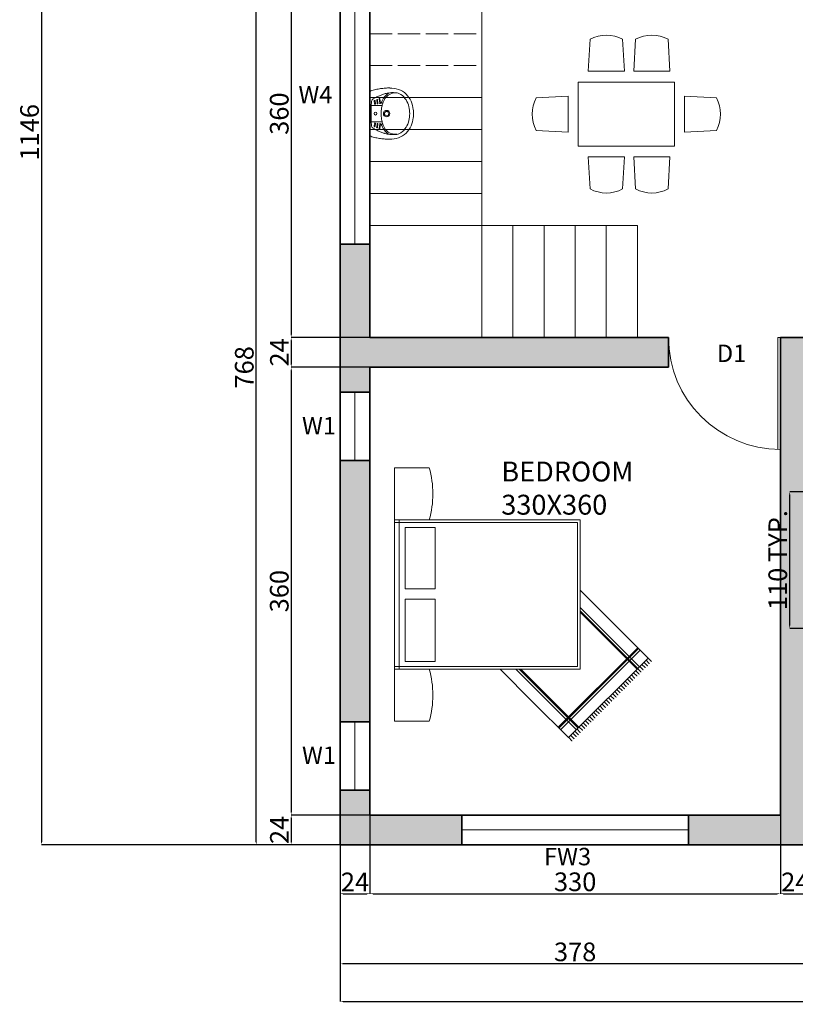
# Model space of a CAD drawing. Units: centimetres. Extents: x 2449 to 7478, y 778 to 2486.
# Tile 1 of 9: x 2449 to 3072, y 940 to 1732. Entities that reach past the tile are written whole.
import ezdxf

# ---------------------------------------------------------------- set-up
doc = ezdxf.new("R2010")
doc.units = ezdxf.units.CM
doc.linetypes.add('ACAD_ISO02W100', pattern=[15, 12, -3])
for name, color, linetype, lineweight in [('0.15', 34, 'Continuous', 15), ('A-ANNO-DIMS', 2, 'Continuous', 18), ('A-ANNO-TEXT', 7, 'Continuous', 18), ('A-AREA-IDEN', 7, 'Continuous', 18), ('A-DOOR', 4, 'Continuous', 18), ('A-FLOR-FIXT', 8, 'Continuous', 18), ('A-FLOR-STRS', 7, 'Continuous', 18), ('A-FLOR-STRS-OVHD', 7, 'ACAD_ISO02W100', 13), ('A-WALL', 7, 'Continuous', 35), ('A-WALL-PATT', 7, 'Continuous', 13), ('B-FURNITURE', 22, 'Continuous', 18), ('Win', 1, 'Continuous', 18)]:
    doc.layers.add(name, color=color, linetype=linetype, lineweight=lineweight)
doc.styles.get("Standard").update_dxf_attribs({"font": 'arial.ttf'})
doc.dimstyles.new('ISO-25', dxfattribs={"dimtxt": 15, "dimasz": 2.5, "dimexe": 0, "dimexo": 0, "dimgap": 0, "dimtad": 1, "dimtxsty": 'Standard', "dimcen": 2.5, "dimadec": 0, "dimazin": 0, "dimtfac": 1, "dimtmove": 0, "dimatfit": 3, "dimfxl": 1, "dimarcsym": 0})

# ---------------------------------------------------------------- blocks, each defined once
blk = doc.blocks.new('table-11')
at = {"color": 0, "linetype": 'ByBlock'}
for p, q in [((-1.122, 0.533), (-1.144, 0.134)), ((-0.716, 0.533), (-0.694, 0.134)), ((-0.554, 0.533), (-0.576, 0.134)), ((-0.148, 0.533), (-0.126, 0.134)), ((-1.144, 0.134), (-0.694, 0.134)), ((-0.576, 0.134), (-0.126, 0.134)), ((0, 0), (-1.2, 0)), ((-1.2, -0.8), (-1.2, 0)), ((0, -0.8), (0, 0)), ((-1.723, -0.197), (-1.324, -0.175)), ((-1.324, -0.625), (-1.324, -0.175)), ((0.523, -0.197), (0.124, -0.175)), ((0.124, -0.625), (0.124, -0.175)), ((-1.723, -0.603), (-1.324, -0.625)), ((0.523, -0.603), (0.124, -0.625)), ((0, -0.8), (-1.2, -0.8)), ((-1.144, -0.934), (-0.694, -0.934)), ((-1.122, -1.333), (-1.144, -0.934)), ((-0.716, -1.333), (-0.694, -0.934)), ((-0.576, -0.934), (-0.126, -0.934)), ((-0.554, -1.333), (-0.576, -0.934)), ((-0.148, -1.333), (-0.126, -0.934))]:
    blk.add_line(p, q, dxfattribs=at)
for centre, start, end in [((-0.919, 0.159), 61.4891, 118.5109), ((-0.351, 0.159), 61.4891, 118.5109), ((-1.349, -0.4), 151.4891, 208.5109), ((0.149, -0.4), 331.4891, 28.5109), ((-0.919, -0.959), 241.4891, 298.5109), ((-0.351, -0.959), 241.4891, 298.5109)]:
    blk.add_arc(centre, 0.425, start, end, dxfattribs=at)
blk = doc.blocks.new('A$C376C2187')
at = {"layer": 'B-FURNITURE'}
for p, q in [((-1.53, 1.82), (-1.53, 2.24)), ((-1.53, 2.24), (-0.9, 2.24)), ((-0.9, 0), (-0.9, 2.24)), ((-0.9, 2.24), (0.9, 2.24)), ((-0.9, 2.24), (-0.9, 1.82)), ((-0.9, 2.182), (0.9, 2.182)), ((-0.87, 0.03), (-0.87, 2.24)), ((0.87, 2.24), (0.87, 0.03)), ((0.9, 2.24), (0.9, 0)), ((0.9, 1.82), (0.9, 2.24)), ((0.9, 2.24), (1.53, 2.24)), ((1.53, 2.24), (1.53, 1.82)), ((-0.807, 2.112), (-0.057, 2.112)), ((-0.807, 1.749), (-0.807, 2.112)), ((-0.057, 2.112), (-0.057, 1.749)), ((0.069, 2.112), (0.807, 2.112)), ((0.069, 2.112), (0.069, 1.749)), ((0.807, 2.112), (0.807, 1.749)), ((-0.807, 1.749), (-0.057, 1.749)), ((0.069, 1.749), (0.807, 1.749)), ((0.9, 0), (-0.9, 0)), ((0.87, 0.03), (-0.87, 0.03))]:
    blk.add_line(p, q, dxfattribs=at)
for centre in [(-1.215, 2.926), (1.215, 2.926)]:
    blk.add_arc(centre, 1.15, 254.0965, 285.9035, dxfattribs=at)
blk = doc.blocks.new('lavamanos 2')
at = {"layer": '0.15'}
for p, q in [((0, 0.234), (0, -0.234)), ((-0.13, 0.11), (-0.131, 0.11)), ((-0.113, 0.112), (-0.107, 0.158)), ((-0.104, 0.111), (-0.098, 0.157)), ((-0.086, 0.109), (-0.081, 0.147)), ((-0.077, 0.107), (-0.072, 0.145)), ((-0.059, 0.105), (-0.055, 0.135)), ((-0.05, 0.104), (-0.046, 0.134)), ((-0.014, 0.087), (-0.13, 0.086)), ((-0.014, -0.087), (-0.13, -0.086)), ((-0.05, -0.104), (-0.046, -0.134)), ((-0.13, -0.11), (-0.131, -0.11)), ((-0.113, -0.112), (-0.107, -0.158)), ((-0.104, -0.111), (-0.098, -0.157)), ((-0.086, -0.109), (-0.081, -0.147)), ((-0.077, -0.107), (-0.072, -0.145)), ((-0.059, -0.105), (-0.055, -0.135))]:
    blk.add_line(p, q, dxfattribs=at)
for centre, radius in [((-0.178, 0), 0.035), ((-0.178, 0), 0.0235), ((-0.06, 0), 0.015)]:
    blk.add_circle(centre, radius, dxfattribs=at)
for centre, radius, start, end in [((-0.242, 0.066), 0.202, 108.1945, 135.3686), ((-0.266, 0.104), 0.119, 92.4774, 122.1411), ((-0.203, -0.086), 0.359, 91.203, 106.4255), ((-0.277, 0.068), 0.153, 57.2491, 95.54), ((-0.244, -0.013), 0.237, 77.2482, 96.4632), ((-0.221, -0.685), 0.959, 86.5514, 89.4131), ((-0.277, 0.068), 0.168, 56.8766, 64.9971), ((-0.222, 0.003), 0.218, 71.9849, 82.0124), ((-0.212, -0.548), 0.82, 83.1224, 86.5796), ((5.828, 30.215), 30.532, 258.7782, 258.876), ((-0.126, -0.066), 0.329, 69.0601, 78.8218), ((-0.02, 0.212), 0.0314, 54.7949, 69.0601), ((-0.005, 0.234), 0.005, 0, 54.7949), ((-0.056, -0.018), 0.411, 158.7011, 171.3102), ((-0.166, 0.001), 0.302, 136.5719, 154.3277), ((-0.2, 0.026), 0.22, 147.1156, 167.4425), ((-0.242, 0.065), 0.164, 121.9929, 150.5889), ((-0.366, -0.002), 0.263, 40.3525, 49.0046), ((-0.366, -0.002), 0.278, 40.3525, 49.2255), ((-0.237, 0.11), 0.0921, 27.3186, 39.1156), ((-0.349, 0.036), 0.226, 22.3361, 30.8927), ((-0.31, -0.315), 0.547, 69.5191, 73.4912), ((-0.237, 0.11), 0.107, 27.5743, 39.1156), ((-0.349, 0.036), 0.241, 22.1921, 30.7838), ((-1.266, -0.239), 1.182, 16.3631, 17.7767), ((-0.132, 0.117), 0.007, 197.4099, 270.4949), ((-0.13, 0.117), 0.007, 270.4949, 17.3953), ((-1.266, -0.239), 1.197, 17.3953, 17.8049), ((-0.299, -0.285), 0.516, 65.23, 69.5378), ((-0.108, 0.111), 0.0045, 172.614, 352.614), ((-0.102, 0.158), 0.0045, 352.614, 172.614), ((-0.081, 0.108), 0.0045, 172.614, 352.614), ((-0.278, -0.241), 0.466, 60.2413, 65.2382), ((-0.076, 0.146), 0.0045, 352.614, 172.614), ((-0.054, 0.104), 0.0045, 172.614, 352.614), ((-0.05, 0.135), 0.0045, 352.614, 172.614), ((-0.065, 0.118), 0.049, 1.5827, 68.6208), ((-2.148, 0.001), 2.135, 359.9754, 3.1901), ((-0.209, 0.006), 0.256, 171.3102, 181.2627), ((-0.209, -0.006), 0.256, 178.7373, 188.6898), ((0.466, -0.083), 0.895, 169.8632, 174.658), ((0.466, 0.083), 0.895, 185.342, 190.1368), ((0.185, 0.165), 0.325, 192.5389, 196.7072), ((0.389, 0.121), 0.517, 185.5053, 189.8131), ((-0.718, -0.007), 0.599, 0.6765, 3.8216), ((-0.718, 0.007), 0.599, 356.1784, 359.3235), ((-2.148, -0.001), 2.135, 356.8099, 0.0246), ((-0.056, 0.018), 0.411, 188.6898, 201.2989), ((-0.2, -0.026), 0.22, 192.5575, 212.8844), ((-1.266, 0.239), 1.182, 342.2233, 343.6369), ((0.185, -0.165), 0.325, 163.2928, 167.4611), ((0.389, -0.121), 0.517, 170.1869, 174.4947), ((-0.081, -0.108), 0.0045, 7.386, 187.386), ((-0.054, -0.104), 0.0045, 7.386, 187.386), ((-0.166, -0.001), 0.302, 205.6723, 223.4281), ((-0.242, -0.066), 0.202, 224.6314, 251.8055), ((-0.242, -0.065), 0.164, 209.4111, 238.0071), ((-0.266, -0.104), 0.119, 237.8589, 267.5226), ((-0.277, -0.068), 0.153, 264.46, 302.7509), ((-0.277, -0.068), 0.168, 295.0029, 303.1234), ((-0.366, 0.002), 0.263, 310.9954, 319.6475), ((-0.222, -0.003), 0.218, 277.9876, 288.0151), ((-0.366, 0.002), 0.278, 310.7745, 319.6475), ((-0.237, -0.11), 0.0921, 320.8844, 332.6814), ((-0.349, -0.036), 0.226, 329.1073, 337.6639), ((-0.31, 0.315), 0.547, 286.5088, 290.4809), ((-0.237, -0.11), 0.107, 320.8844, 332.4257), ((-0.349, -0.036), 0.241, 329.2162, 337.8079), ((-0.132, -0.117), 0.007, 89.5051, 162.5901), ((-0.13, -0.117), 0.007, 342.6047, 89.5051), ((-1.266, 0.239), 1.197, 342.1951, 342.6047), ((-0.299, 0.286), 0.516, 290.4622, 294.77), ((-0.108, -0.111), 0.0045, 7.386, 187.386), ((-0.102, -0.158), 0.0045, 187.386, 7.386), ((-0.278, 0.241), 0.466, 294.7618, 299.7587), ((-0.076, -0.146), 0.0045, 187.386, 7.386), ((-0.05, -0.135), 0.0045, 187.386, 7.386), ((-0.065, -0.118), 0.049, 291.3792, 358.4173), ((-0.203, 0.086), 0.359, 253.5745, 268.797), ((-0.244, 0.013), 0.237, 263.5368, 282.7518), ((-0.221, 0.685), 0.959, 270.5869, 273.4486), ((-0.212, 0.548), 0.82, 273.4204, 276.8776), ((5.828, -30.215), 30.532, 101.124, 101.2218), ((-0.126, 0.066), 0.329, 281.1782, 290.9399), ((-0.02, -0.212), 0.0314, 290.9399, 305.2051), ((-0.005, -0.234), 0.005, 305.2051, 0)]:
    blk.add_arc(centre, radius, start, end, dxfattribs=at)
blk = doc.blocks.new('*D32')
at = {"layer": 'A-ANNO-DIMS', "color": 0, "lineweight": -2, "transparency": 16777216}
for p, q in [((2706.09, 1836.34), (2666.8, 1836.34)), ((2666.8, 1833.84), (2666.8, 1478.84)), ((2730.09, 1476.34), (2666.8, 1476.34))]:
    blk.add_line(p, q, dxfattribs=at)
at = {"layer": 'A-ANNO-DIMS', "color": 0, "transparency": 16777216}
for points in [[(2666.38, 1833.84), (2667.22, 1833.84), (2666.8, 1836.34)], [(2666.38, 1478.84), (2667.22, 1478.84), (2666.8, 1476.34)]]:
    blk.add_solid(points, dxfattribs=at)
at = {"layer": 'Defpoints', "color": 0, "transparency": 16777216}
for p in [(2706.09, 1836.34), (2666.8, 1476.34), (2730.09, 1476.34)]:
    blk.add_point(p, dxfattribs=at)
at = {"layer": 'A-ANNO-DIMS', "color": 0, "transparency": 16777216, "insert": (2659.14, 1656.34), "char_height": 15, "attachment_point": 5, "rotation": 90}
blk.add_mtext('360', dxfattribs=at)
blk = doc.blocks.new('*D33')
at = {"layer": 'A-ANNO-DIMS', "color": 0, "lineweight": -2, "transparency": 16777216}
for p, q in [((2730.09, 1476.34), (2666.8, 1476.34)), ((2666.8, 1473.84), (2666.8, 1454.84)), ((2730.09, 1452.34), (2666.8, 1452.34))]:
    blk.add_line(p, q, dxfattribs=at)
at = {"layer": 'A-ANNO-DIMS', "color": 0, "transparency": 16777216}
for points in [[(2666.38, 1473.84), (2667.22, 1473.84), (2666.8, 1476.34)], [(2666.38, 1454.84), (2667.22, 1454.84), (2666.8, 1452.34)]]:
    blk.add_solid(points, dxfattribs=at)
at = {"layer": 'Defpoints', "color": 0, "transparency": 16777216}
for p in [(2730.09, 1476.34), (2666.8, 1452.34), (2730.09, 1452.34)]:
    blk.add_point(p, dxfattribs=at)
at = {"layer": 'A-ANNO-DIMS', "color": 0, "transparency": 16777216, "insert": (2659.27, 1464.34), "char_height": 15, "attachment_point": 5, "rotation": 90}
blk.add_mtext('24', dxfattribs=at)
blk = doc.blocks.new('*D34')
at = {"layer": 'A-ANNO-DIMS', "color": 0, "lineweight": -2, "transparency": 16777216}
for p, q in [((2730.09, 1452.34), (2666.8, 1452.34)), ((2666.8, 1449.84), (2666.8, 1094.84)), ((2730.09, 1092.34), (2666.8, 1092.34))]:
    blk.add_line(p, q, dxfattribs=at)
at = {"layer": 'A-ANNO-DIMS', "color": 0, "transparency": 16777216}
for points in [[(2666.38, 1449.84), (2667.22, 1449.84), (2666.8, 1452.34)], [(2666.38, 1094.84), (2667.22, 1094.84), (2666.8, 1092.34)]]:
    blk.add_solid(points, dxfattribs=at)
at = {"layer": 'Defpoints', "color": 0, "transparency": 16777216}
for p in [(2730.09, 1452.34), (2666.8, 1092.34), (2730.09, 1092.34)]:
    blk.add_point(p, dxfattribs=at)
at = {"layer": 'A-ANNO-DIMS', "color": 0, "transparency": 16777216, "insert": (2659.14, 1272.34), "char_height": 15, "attachment_point": 5, "rotation": 90}
blk.add_mtext('360', dxfattribs=at)
blk = doc.blocks.new('*D35')
at = {"layer": 'A-ANNO-DIMS', "color": 0, "lineweight": -2, "transparency": 16777216}
for p, q in [((2730.09, 1092.34), (2666.8, 1092.34)), ((2666.8, 1089.84), (2666.8, 1070.84)), ((2706.09, 1068.34), (2666.8, 1068.34))]:
    blk.add_line(p, q, dxfattribs=at)
at = {"layer": 'A-ANNO-DIMS', "color": 0, "transparency": 16777216}
for points in [[(2666.38, 1089.84), (2667.22, 1089.84), (2666.8, 1092.34)], [(2666.38, 1070.84), (2667.22, 1070.84), (2666.8, 1068.34)]]:
    blk.add_solid(points, dxfattribs=at)
at = {"layer": 'Defpoints', "color": 0, "transparency": 16777216}
for p in [(2730.09, 1092.34), (2666.8, 1068.34), (2706.09, 1068.34)]:
    blk.add_point(p, dxfattribs=at)
at = {"layer": 'A-ANNO-DIMS', "color": 0, "transparency": 16777216, "insert": (2659.27, 1080.34), "char_height": 15, "attachment_point": 5, "rotation": 90}
blk.add_mtext('24', dxfattribs=at)
blk = doc.blocks.new('*D36')
at = {"layer": 'A-ANNO-DIMS', "color": 0, "lineweight": -2, "transparency": 16777216}
for p, q in [((2706.09, 1836.34), (2638.68, 1836.34)), ((2638.68, 1070.84), (2638.68, 1833.84)), ((2706.09, 1068.34), (2638.68, 1068.34))]:
    blk.add_line(p, q, dxfattribs=at)
at = {"layer": 'A-ANNO-DIMS', "color": 0, "transparency": 16777216}
for points in [[(2638.26, 1833.84), (2639.09, 1833.84), (2638.68, 1836.34)], [(2638.26, 1070.84), (2639.09, 1070.84), (2638.68, 1068.34)]]:
    blk.add_solid(points, dxfattribs=at)
at = {"layer": 'Defpoints', "color": 0, "transparency": 16777216}
for p in [(2638.68, 1836.34), (2706.09, 1836.34), (2706.09, 1068.34)]:
    blk.add_point(p, dxfattribs=at)
at = {"layer": 'A-ANNO-DIMS', "color": 0, "transparency": 16777216, "insert": (2631.02, 1452.34), "char_height": 15, "attachment_point": 5, "rotation": 90}
blk.add_mtext('768', dxfattribs=at)
blk = doc.blocks.new('*D38')
at = {"layer": 'A-ANNO-DIMS', "color": 0, "lineweight": -2, "transparency": 16777216}
for p, q in [((2578.09, 2214.34), (2466.02, 2214.34)), ((2466.02, 2211.84), (2466.02, 1070.84)), ((2706.09, 1068.34), (2466.02, 1068.34))]:
    blk.add_line(p, q, dxfattribs=at)
at = {"layer": 'A-ANNO-DIMS', "color": 0, "transparency": 16777216}
for points in [[(2465.6, 2211.84), (2466.43, 2211.84), (2466.02, 2214.34)], [(2465.6, 1070.84), (2466.43, 1070.84), (2466.02, 1068.34)]]:
    blk.add_solid(points, dxfattribs=at)
at = {"layer": 'Defpoints', "color": 0, "transparency": 16777216}
for p in [(2578.09, 2214.34), (2466.02, 1068.34), (2706.09, 1068.34)]:
    blk.add_point(p, dxfattribs=at)
at = {"layer": 'A-ANNO-DIMS', "color": 0, "transparency": 16777216, "insert": (2458.36, 1641.34), "char_height": 15, "attachment_point": 5, "rotation": 90}
blk.add_mtext('1146', dxfattribs=at)
blk = doc.blocks.new('*D39')
at = {"layer": 'A-ANNO-DIMS', "color": 0, "lineweight": -2, "transparency": 16777216}
for p, q in [((2706.09, 1092.34), (2706.09, 1029.04)), ((2730.09, 1092.34), (2730.09, 1029.04)), ((2708.59, 1029.04), (2727.59, 1029.04))]:
    blk.add_line(p, q, dxfattribs=at)
at = {"layer": 'A-ANNO-DIMS', "color": 0, "transparency": 16777216}
for points in [[(2708.59, 1029.46), (2708.59, 1028.62), (2706.09, 1029.04)], [(2727.59, 1029.46), (2727.59, 1028.62), (2730.09, 1029.04)]]:
    blk.add_solid(points, dxfattribs=at)
at = {"layer": 'Defpoints', "color": 0, "transparency": 16777216}
for p in [(2706.09, 1092.34), (2730.09, 1092.34), (2730.09, 1029.04)]:
    blk.add_point(p, dxfattribs=at)
at = {"layer": 'A-ANNO-DIMS', "color": 0, "transparency": 16777216, "insert": (2718.09, 1036.57), "char_height": 15, "attachment_point": 5}
blk.add_mtext('24', dxfattribs=at)
blk = doc.blocks.new('*D40')
at = {"layer": 'A-ANNO-DIMS', "color": 0, "lineweight": -2, "transparency": 16777216}
for p, q in [((2730.09, 1092.34), (2730.09, 1029.04)), ((3060.09, 1092.34), (3060.09, 1029.04)), ((2732.59, 1029.04), (3057.59, 1029.04))]:
    blk.add_line(p, q, dxfattribs=at)
at = {"layer": 'A-ANNO-DIMS', "color": 0, "transparency": 16777216}
for points in [[(2732.59, 1029.46), (2732.59, 1028.62), (2730.09, 1029.04)], [(3057.59, 1029.46), (3057.59, 1028.62), (3060.09, 1029.04)]]:
    blk.add_solid(points, dxfattribs=at)
at = {"layer": 'Defpoints', "color": 0, "transparency": 16777216}
for p in [(2730.09, 1092.34), (3060.09, 1092.34), (3060.09, 1029.04)]:
    blk.add_point(p, dxfattribs=at)
at = {"layer": 'A-ANNO-DIMS', "color": 0, "transparency": 16777216, "insert": (2895.09, 1036.7), "char_height": 15, "attachment_point": 5}
blk.add_mtext('330', dxfattribs=at)
blk = doc.blocks.new('*D41')
at = {"layer": 'A-ANNO-DIMS', "color": 0, "lineweight": -2, "transparency": 16777216}
for p, q in [((3060.09, 1092.34), (3060.09, 1029.04)), ((3084.09, 1068.34), (3084.09, 1029.04)), ((3062.59, 1029.04), (3081.59, 1029.04))]:
    blk.add_line(p, q, dxfattribs=at)
at = {"layer": 'A-ANNO-DIMS', "color": 0, "transparency": 16777216}
for points in [[(3062.59, 1029.46), (3062.59, 1028.62), (3060.09, 1029.04)], [(3081.59, 1029.46), (3081.59, 1028.62), (3084.09, 1029.04)]]:
    blk.add_solid(points, dxfattribs=at)
at = {"layer": 'Defpoints', "color": 0, "transparency": 16777216}
for p in [(3060.09, 1092.34), (3084.09, 1068.34), (3084.09, 1029.04)]:
    blk.add_point(p, dxfattribs=at)
at = {"layer": 'A-ANNO-DIMS', "color": 0, "transparency": 16777216, "insert": (3072.09, 1036.57), "char_height": 15, "attachment_point": 5}
blk.add_mtext('24', dxfattribs=at)
blk = doc.blocks.new('*D56')
at = {"layer": 'A-ANNO-DIMS', "color": 0, "lineweight": -2, "transparency": 16777216}
for p, q in [((2706.09, 1068.34), (2706.09, 972.69)), ((3084.09, 1068.34), (3084.09, 972.69)), ((3081.59, 972.69), (2708.59, 972.69))]:
    blk.add_line(p, q, dxfattribs=at)
at = {"layer": 'A-ANNO-DIMS', "color": 0, "transparency": 16777216}
for points in [[(2708.59, 973.11), (2708.59, 972.27), (2706.09, 972.69)], [(3081.59, 973.11), (3081.59, 972.27), (3084.09, 972.69)]]:
    blk.add_solid(points, dxfattribs=at)
at = {"layer": 'Defpoints', "color": 0, "transparency": 16777216}
for p in [(2706.09, 1068.34), (3084.09, 1068.34), (2706.09, 972.69)]:
    blk.add_point(p, dxfattribs=at)
at = {"layer": 'A-ANNO-DIMS', "color": 0, "transparency": 16777216, "insert": (2895.09, 980.35), "char_height": 15, "attachment_point": 5}
blk.add_mtext('378', dxfattribs=at)
blk = doc.blocks.new('*D57')
at = {"layer": 'A-ANNO-DIMS', "color": 0, "lineweight": -2, "transparency": 16777216}
for p, q in [((2706.09, 1068.34), (2706.09, 942.3)), ((3812.09, 1044.34), (3812.09, 942.3)), ((2708.59, 942.3), (3809.59, 942.3))]:
    blk.add_line(p, q, dxfattribs=at)
at = {"layer": 'A-ANNO-DIMS', "color": 0, "transparency": 16777216}
for points in [[(2708.59, 942.72), (2708.59, 941.88), (2706.09, 942.3)], [(3809.59, 942.72), (3809.59, 941.88), (3812.09, 942.3)]]:
    blk.add_solid(points, dxfattribs=at)
at = {"layer": 'Defpoints', "color": 0, "transparency": 16777216}
for p in [(2706.09, 1068.34), (3812.09, 1044.34), (3812.09, 942.3)]:
    blk.add_point(p, dxfattribs=at)
at = {"layer": 'A-ANNO-DIMS', "color": 0, "transparency": 16777216, "insert": (3259.09, 949.96), "char_height": 15, "attachment_point": 5}
blk.add_mtext('1106', dxfattribs=at)
blk = doc.blocks.new('2')
for p, q in [((5717.35, 1812.71), (5717.35, 1722.71)), ((5719.35, 1812.71), (5719.35, 1722.71)), ((5719.35, 1722.71), (5717.35, 1722.71))]:
    blk.add_line(p, q)
blk.add_arc((5717.35, 1722.71), 90, 0, 90)
blk = doc.blocks.new('RUG-FRINGED-B')
for p, q in [((90.45, 95.22), (64.35, 121.32)), ((64.35, 107.43), (83.5, 88.28)), ((64.35, 104.72), (82.15, 86.92)), ((64.35, 103.56), (81.57, 86.34)), ((90.45, 95.22), (119.07, 66.61)), ((112.12, 59.66), (83.5, 88.28)), ((110.18, 57.73), (81.57, 86.34)), ((110.76, 58.31), (82.15, 86.92)), ((110.74, 74.93), (46.79, 10.99)), ((111.32, 74.35), (47.37, 10.4)), ((112.68, 73), (48.73, 9.05)), ((119.07, 66.61), (55.12, 2.66)), ((117.39, 64.93), (120.01, 62.3)), ((119.07, 66.61), (121.69, 63.98)), ((0, 57.78), (26.5, 31.28)), ((32.89, 37.67), (12.78, 57.78)), ((34.25, 39.02), (15.49, 57.78)), ((34.83, 39.6), (16.65, 57.78)), ((108.98, 56.53), (111.61, 53.9)), ((110.66, 58.21), (113.29, 55.58)), ((112.34, 59.89), (114.97, 57.26)), ((114.02, 61.57), (116.65, 58.94)), ((115.7, 63.25), (118.33, 60.62)), ((100.58, 48.13), (103.21, 45.5)), ((102.26, 49.81), (104.89, 47.18)), ((103.94, 51.49), (106.57, 48.86)), ((105.62, 53.17), (108.25, 50.54)), ((107.3, 54.85), (109.93, 52.22)), ((34.83, 39.6), (63.44, 10.99)), ((92.18, 39.73), (94.81, 37.1)), ((93.86, 41.41), (96.49, 38.78)), ((95.54, 43.09), (98.17, 40.46)), ((97.22, 44.77), (99.85, 42.14)), ((98.9, 46.45), (101.53, 43.82)), ((32.89, 37.67), (61.51, 9.05)), ((34.25, 39.02), (62.86, 10.4)), ((85.46, 33.01), (88.09, 30.38)), ((87.14, 34.69), (89.77, 32.06)), ((88.82, 36.37), (91.45, 33.74)), ((90.5, 38.05), (93.13, 35.42)), ((55.12, 2.66), (26.5, 31.28)), ((77.06, 24.61), (79.69, 21.98)), ((78.74, 26.29), (81.37, 23.66)), ((80.42, 27.97), (83.05, 25.34)), ((82.1, 29.65), (84.73, 27.02)), ((83.78, 31.33), (86.41, 28.7)), ((68.66, 16.21), (71.29, 13.58)), ((70.34, 17.89), (72.97, 15.26)), ((72.02, 19.57), (74.65, 16.94)), ((73.7, 21.25), (76.33, 18.62)), ((75.38, 22.93), (78.01, 20.3)), ((61.94, 9.48), (64.57, 6.86)), ((63.62, 11.17), (66.25, 8.54)), ((65.3, 12.85), (67.93, 10.22)), ((66.98, 14.53), (69.61, 11.9)), ((55.22, 2.76), (57.85, 0.14)), ((56.9, 4.44), (59.53, 1.82)), ((58.58, 6.12), (61.21, 3.5)), ((60.26, 7.8), (62.89, 5.18))]:
    blk.add_line(p, q)
for centre in [(121.75, 63.92), (113.35, 55.52), (115.03, 57.2), (116.71, 58.88), (118.39, 60.56), (120.07, 62.24), (106.63, 48.8), (108.31, 50.48), (109.99, 52.16), (111.67, 53.84), (98.23, 40.4), (99.91, 42.08), (101.59, 43.76), (103.27, 45.44), (104.95, 47.12), (89.83, 32), (91.51, 33.68), (93.19, 35.36), (94.87, 37.04), (96.55, 38.72), (83.11, 25.28), (84.79, 26.96), (86.47, 28.64), (88.15, 30.32), (74.71, 16.88), (76.39, 18.56), (78.07, 20.24), (79.75, 21.92), (81.43, 23.6), (66.31, 8.48), (67.99, 10.16), (69.67, 11.84), (71.35, 13.52), (73.03, 15.2), (57.91, 0.08), (59.59, 1.76), (61.27, 3.44), (62.95, 5.12), (64.63, 6.8)]:
    blk.add_circle(centre, 0.0789)
blk = doc.blocks.new('*D73')
at = {"layer": 'A-ANNO-DIMS', "color": 0, "lineweight": -2, "transparency": 16777216}
for p, q in [((3084.09, 1352.34), (3067.59, 1352.34)), ((3067.59, 1244.84), (3067.59, 1349.84)), ((3084.09, 1242.34), (3067.59, 1242.34))]:
    blk.add_line(p, q, dxfattribs=at)
at = {"layer": 'A-ANNO-DIMS', "color": 0, "transparency": 16777216}
for points in [[(3067.17, 1349.84), (3068, 1349.84), (3067.59, 1352.34)], [(3067.17, 1244.84), (3068, 1244.84), (3067.59, 1242.34)]]:
    blk.add_solid(points, dxfattribs=at)
at = {"layer": 'Defpoints', "color": 0, "transparency": 16777216}
for p in [(3067.59, 1352.34), (3084.09, 1352.34), (3084.09, 1242.34)]:
    blk.add_point(p, dxfattribs=at)
at = {"layer": 'A-ANNO-DIMS', "color": 0, "transparency": 16777216, "insert": (3059.93, 1297.34), "char_height": 15, "attachment_point": 5, "rotation": 90}
blk.add_mtext('110 TYP.', dxfattribs=at)

msp = doc.modelspace()

# ---------------------------------------------------------------- hatches: boundary and pattern name
at = {"layer": 'A-WALL-PATT'}
h = msp.add_hatch(color=256, dxfattribs=at)
h.dxf.hatch_style = 1
h.paths.add_polyline_path([(3060.088, 1092.34), (2986.088, 1092.34), (2986.088, 1068.34), (3084.088, 1068.34), (3084.088, 1476.34), (3060.088, 1476.34)])
h.paths.add_polyline_path([(2706.088, 1167.34), (2730.088, 1167.34), (2730.088, 1377.34), (2706.088, 1377.34)])
h.paths.add_polyline_path([(2804.088, 1068.34), (2804.088, 1092.34), (2730.088, 1092.34), (2730.088, 1112.34), (2706.088, 1112.34), (2706.088, 1068.34)])
h.paths.add_polyline_path([(2730.088, 1551.34), (2706.088, 1551.34), (2706.088, 1432.34), (2730.088, 1432.34), (2730.088, 1452.34), (2970.088, 1452.34), (2970.088, 1476.34), (2730.088, 1476.34)])
h.paths.add_polyline_path([(3434.088, 1654.34), (3434.088, 1266.34), (3405.088, 1266.34), (3405.088, 1242.34), (3458.088, 1242.34), (3458.088, 1404.34), (3482.088, 1404.34), (3482.088, 1428.34), (3458.088, 1428.34), (3458.088, 1678.34), (3260.088, 1678.34), (3260.088, 1654.34)])
h.paths.add_polyline_path([(3223.088, 1266.34), (3194.088, 1266.34), (3194.088, 1242.34), (3223.088, 1242.34)])
h.paths.add_polyline_path([(3812.088, 1506.339), (3788.088, 1506.339), (3788.088, 1428.34), (3764.088, 1428.34), (3764.088, 1404.34), (3812.088, 1404.34)])
h.paths.add_polyline_path([(3709.088, 1404.34), (3709.088, 1428.34), (3537.088, 1428.34), (3537.088, 1404.34)])
h.paths.add_polyline_path([(3788.088, 1688.339), (3812.088, 1688.339), (3812.088, 1826.34), (3788.088, 1826.34), (3788.088, 1792.34), (3647.088, 1792.34), (3647.088, 1768.34), (3788.088, 1768.34)])
h.paths.add_polyline_path([(3788.088, 1956.34), (3548.088, 1956.34), (3548.088, 1792.34), (3434.088, 1792.34), (3434.088, 1768.34), (3572.088, 1768.34), (3572.088, 1932.34), (3788.088, 1932.34), (3788.088, 1898.34), (3812.088, 1898.34), (3812.088, 2065.339), (3788.088, 2065.339)])
h.paths.add_polyline_path([(3788.088, 2358.34), (3788.088, 2247.339), (3812.088, 2247.339), (3812.088, 2382.34), (3764.088, 2382.34), (3764.088, 2358.34)])
h.paths.add_polyline_path([(3537.088, 2382.34), (3537.088, 2358.34), (3709.088, 2358.34), (3709.088, 2382.34)])
h.paths.add_polyline_path([(3458.088, 2358.34), (3482.088, 2358.34), (3482.088, 2382.34), (3434.088, 2382.34), (3434.088, 2214.34), (3395.088, 2214.34), (3395.088, 2190.34), (3434.088, 2190.34), (3434.088, 2065.34), (3458.088, 2065.34)])
h.paths.add_polyline_path([(3231.088, 2214.34), (3231.088, 2190.34), (3260.088, 2190.34), (3260.088, 1966.34), (3434.088, 1966.34), (3434.088, 1932.34), (3458.088, 1932.34), (3458.088, 1990.34), (3284.088, 1990.34), (3284.088, 2190.34), (3323.088, 2190.34), (3323.088, 2214.34)])
h.paths.add_polyline_path([(3130.088, 2190.34), (3159.088, 2190.34), (3159.088, 2214.34), (3032.088, 2214.34), (3032.088, 2190.34), (3106.088, 2190.34), (3106.088, 1836.34), (3130.088, 1836.34), (3130.088, 1966.34), (3185.088, 1966.34), (3185.088, 1990.34), (3130.088, 1990.34)])
h.paths.add_polyline_path([(2738.088, 2214.34), (2738.088, 2190.34), (2752.088, 2190.34), (2752.088, 1935.34), (2776.088, 1935.34), (2776.088, 2190.34), (2850.088, 2190.34), (2850.088, 2214.34)])
h.paths.add_polyline_path([(2578.088, 2152.839), (2602.088, 2152.839), (2602.088, 2190.34), (2616.088, 2190.34), (2616.088, 2214.34), (2578.088, 2214.34)])
h.paths.add_polyline_path([(2578.088, 1935.34), (2602.088, 1935.34), (2602.088, 1970.839), (2578.088, 1970.839)])
h.paths.add_polyline_path([(2706.088, 1836.34), (2706.088, 1791.34), (2730.088, 1791.34), (2730.088, 1836.34), (3016.088, 1836.34), (3016.088, 1860.34), (2578.088, 1860.34), (2578.088, 1836.34)])

# ---------------------------------------------------------------- linework, layer by layer
at = {"layer": 'A-FLOR-STRS'}
for p, q in [((2820.088, 1836.34), (2820.088, 1476.34)), ((2730.088, 1669.21), (2820.088, 1669.21)), ((2730.088, 1643.47), (2820.088, 1643.47)), ((2730.088, 1617.76), (2820.088, 1617.76)), ((2730.088, 1592.05), (2820.088, 1592.05)), ((2730.088, 1566.34), (2945.088, 1566.34)), ((2845.088, 1566.34), (2845.088, 1476.34)), ((2870.088, 1566.34), (2870.088, 1476.34)), ((2895.088, 1566.34), (2895.088, 1476.34)), ((2920.088, 1566.34), (2920.088, 1476.34)), ((2945.088, 1566.34), (2945.088, 1476.34))]:
    msp.add_line(p, q, dxfattribs=at)
at = {"layer": 'A-FLOR-STRS-OVHD', "ltscale": 1.5}
for p, q in [((2730.088, 1720.63), (2820.088, 1720.63)), ((2730.088, 1694.92), (2820.088, 1694.92))]:
    msp.add_line(p, q, dxfattribs=at)
at = {"layer": 'A-WALL'}
for p, q in [((2706.088, 1836.34), (2706.088, 1068.34)), ((2730.088, 1836.34), (2730.088, 1476.34)), ((2730.088, 1551.34), (2706.088, 1551.34)), ((2730.088, 1476.34), (2970.088, 1476.34)), ((2970.088, 1476.34), (2970.088, 1452.34)), ((3060.088, 1476.34), (3060.088, 1092.34)), ((3060.088, 1476.34), (3084.088, 1476.34)), ((2730.088, 1452.34), (2970.088, 1452.34)), ((2730.088, 1452.34), (2730.088, 1092.34)), ((2706.088, 1432.34), (2730.088, 1432.34)), ((2706.088, 1377.34), (2730.088, 1377.34)), ((2706.088, 1167.34), (2730.088, 1167.34)), ((2706.088, 1112.34), (2730.088, 1112.34)), ((2730.088, 1092.34), (3060.088, 1092.34)), ((2804.088, 1092.34), (2804.088, 1068.34)), ((2986.088, 1092.34), (2986.088, 1068.34)), ((2706.088, 1068.34), (3458.088, 1068.34))]:
    msp.add_line(p, q, dxfattribs=at)
at = {"layer": 'Win'}
for p, q in [((2718.088, 1791.34), (2718.088, 1551.34)), ((2718.088, 1432.34), (2718.088, 1377.34)), ((2718.088, 1112.34), (2718.088, 1167.34)), ((2804.088, 1080.34), (2986.088, 1080.34))]:
    msp.add_line(p, q, dxfattribs=at)

# ---------------------------------------------------------------- block references
at = {"layer": 'A-DOOR', "rotation": 180}
msp.add_blockref('2', (8777.438, 3199.054), dxfattribs=at)
at = {"layer": 'A-FLOR-FIXT', "xscale": 75.44223598555656, "yscale": 75.44223598555656, "zscale": 75.44223598555656, "rotation": 179.99990349049}
msp.add_blockref('lavamanos 2', (2730.088, 1656.34), dxfattribs=at)
at = {"layer": 'B-FURNITURE'}
for name, p, xscale, yscale, zscale, rotation in [('table-11', (2897.534, 1630.173), 64.48907140530227, 64.48907140530227, 64.48907140530227, 180), ('A$C376C2187', (2899.037, 1269.652), 66.63496932822166, 66.63496932822166, 66.63496932822166, 90)]:
    msp.add_blockref(name, p, dxfattribs=dict(at, xscale=xscale, yscale=yscale, zscale=zscale, rotation=rotation))
msp.add_blockref('RUG-FRINGED-B', (2834.684, 1151.901), dxfattribs=at)

# ---------------------------------------------------------------- texts
at = {"layer": 'A-ANNO-TEXT', "char_height": 14, "attachment_point": 1}
for s, insert in [('{\\fTimes New Roman|b0|i0|c0|p18;\\PW4}', (2672.612, 1701.978)), ('{\\fTimes New Roman|b0|i0|c0|p18;\\PD1}', (3008.97, 1493.941)), ('{\\fTimes New Roman|b0|i0|c0|p18;\\PW1}', (2675.476, 1435.743)), ('{\\fTimes New Roman|b0|i0|c0|p18;\\PW1}', (2675.476, 1170.743)), ('{\\fTimes New Roman|b0|i0|c0|p18;\\PFW3}', (2870.026, 1089.247))]:
    msp.add_mtext_dynamic_manual_height_columns(s, width=211.90348, gutter_width=12.5, heights=[0], dxfattribs=dict(at, insert=insert))
at = {"layer": 'A-AREA-IDEN', "insert": (2835.702, 1403.202), "char_height": 16, "attachment_point": 1}
msp.add_mtext_dynamic_manual_height_columns('{\\fTimes New Roman|b0|i0|c0|p18;\\PBEDROOM           330X360}', width=211.90348, gutter_width=12.5, heights=[0], dxfattribs=at)

# ---------------------------------------------------------------- dimensions: what is measured, and where the dimension line sits
at = {"layer": 'A-ANNO-DIMS'}
for base, p1, p2, override, picture, middle in [((2466.017, 1068.34), (2578.088, 2214.34), (2706.088, 1068.34), {"dimclrd": 0, "dimclre": 0, "dimclrt": 0}, '*D38', (2458.358, 1641.34)), ((2638.677, 1836.34), (2706.088, 1068.34), (2706.088, 1836.34), {"dimclrd": 0, "dimclre": 0, "dimclrt": 0}, '*D36', (2631.018, 1452.34)), ((2666.799, 1476.34), (2706.088, 1836.34), (2730.088, 1476.34), {"dimclrd": 0, "dimclre": 0, "dimclrt": 0}, '*D32', (2659.135, 1656.34)), ((2666.799, 1452.34), (2730.088, 1476.34), (2730.088, 1452.34), {"dimclrd": 0, "dimclre": 0, "dimclrt": 0, "dimtmove": 1}, '*D33', (2659.268, 1464.34)), ((2666.799, 1092.34), (2730.088, 1452.34), (2730.088, 1092.34), {"dimclrd": 0, "dimclre": 0, "dimclrt": 0, "dimtmove": 1}, '*D34', (2659.135, 1272.34)), ((2666.799, 1068.34), (2730.088, 1092.34), (2706.088, 1068.34), {"dimclrd": 0, "dimclre": 0, "dimclrt": 0, "dimtmove": 1}, '*D35', (2659.268, 1080.34))]:
    dim = msp.add_linear_dim(base=base, p1=p1, p2=p2, angle=90, dimstyle='ISO-25', override=override, dxfattribs=at)
    dim.commit()
    dim.dimension.update_dxf_attribs({"geometry": picture, "text_midpoint": middle})
dim = msp.add_linear_dim(base=(3067.588, 1352.34), p1=(3084.088, 1242.34), p2=(3084.088, 1352.34), angle=90, text='<> TYP.', dimstyle='ISO-25', override={"dimdec": 0, "dimlfac": 1, "dimrnd": 0, "dimzin": 0, "dimdsep": 46, "dimlunit": 2}, dxfattribs=at)
dim.commit()
dim.dimension.update_dxf_attribs({"geometry": '*D73', "text_midpoint": (3059.93, 1297.34)})
for base, p1, p2, override, picture, middle in [((2730.088, 1029.039), (2706.088, 1092.34), (2730.088, 1092.34), {"dimclrd": 0, "dimclre": 0, "dimclrt": 0}, '*D39', (2718.088, 1036.569)), ((3060.088, 1029.039), (2730.088, 1092.34), (3060.088, 1092.34), {"dimclrd": 0, "dimclre": 0, "dimclrt": 0, "dimtmove": 1}, '*D40', (2895.088, 1036.702)), ((3084.088, 1029.039), (3060.088, 1092.34), (3084.088, 1068.34), {"dimclrd": 0, "dimclre": 0, "dimclrt": 0, "dimtmove": 1}, '*D41', (3072.088, 1036.569)), ((2706.088, 972.69), (3084.088, 1068.34), (2706.088, 1068.34), {"dimclrd": 0, "dimclre": 0, "dimclrt": 0, "dimtmove": 1}, '*D56', (2895.088, 980.354)), ((3812.088, 942.302), (2706.088, 1068.34), (3812.088, 1044.34), {"dimclrd": 0, "dimclre": 0, "dimclrt": 0}, '*D57', (3259.088, 949.96))]:
    dim = msp.add_linear_dim(base=base, p1=p1, p2=p2, dimstyle='ISO-25', override=override, dxfattribs=at)
    dim.commit()
    dim.dimension.update_dxf_attribs({"geometry": picture, "text_midpoint": middle})

doc.saveas('drawing.dxf')
